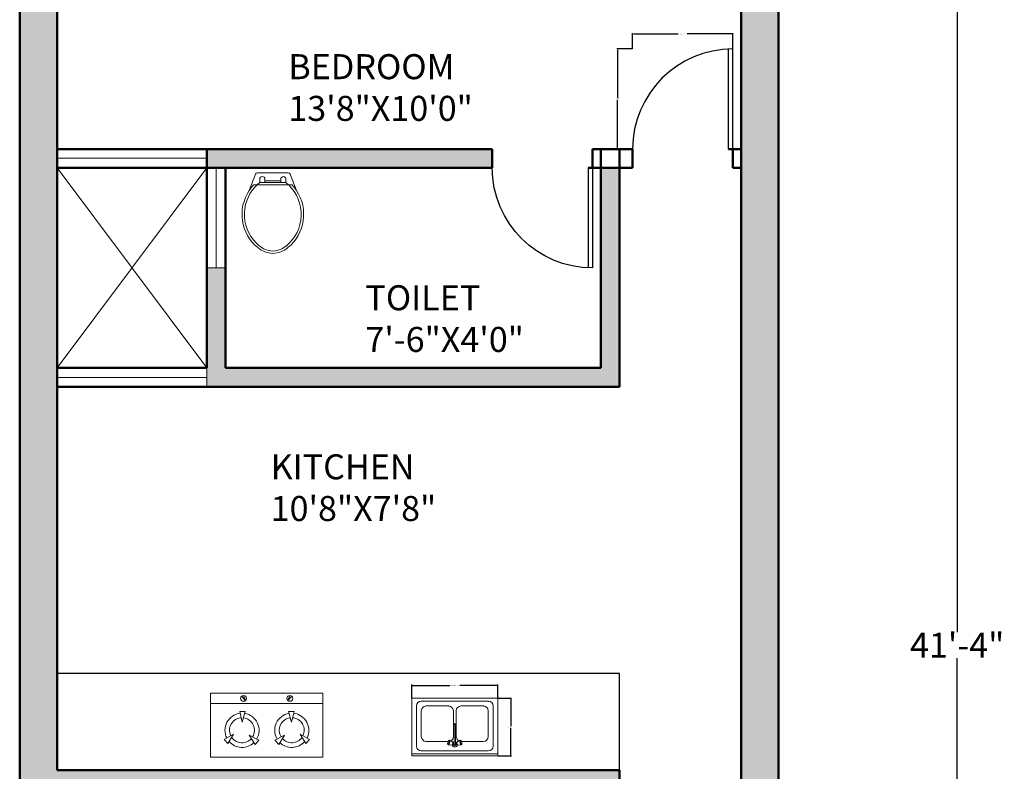
# Model space of a CAD drawing. Units: inches. Extents: x 3 to 485, y -522 to 42.
# Tile 5 of 6: x 249 to 485, y -264 to -84. Entities that reach past the tile are written whole.
import ezdxf

# ---------------------------------------------------------------- set-up
doc = ezdxf.new("R2010")
doc.units = ezdxf.units.IN
doc.header["$MEASUREMENT"] = 0
for name, color, linetype, lineweight in [('A-ANNO-DIMS', 2, 'Continuous', 18), ('A-AREA-IDEN', 7, 'Continuous', 18), ('A-DOOR', 3, 'Continuous', 25), ('A-EQPM', 8, 'Continuous', 18), ('A-FLOR-CASE', 8, 'Continuous', 25), ('A-FLOR-FIXT', 9, 'Continuous', 18), ('A-FLOR-OPEN', 8, 'Continuous', 18), ('A-GLAZ', 4, 'Continuous', 18), ('A-WALL', 7, 'Continuous', 50)]:
    doc.layers.add(name, color=color, linetype=linetype, lineweight=lineweight)
doc.layers.add('A-WALL-PATT', color=18, linetype='Continuous', lineweight=13, true_color=0x000000)
doc.styles.get("Standard").update_dxf_attribs({"font": 'arial.ttf'})
doc.dimstyles.get("Standard").update_dxf_attribs({"dimtxt": 0.18, "dimasz": 0.18, "dimexe": 0.18, "dimexo": 0.0625, "dimgap": 0.09, "dimtad": 0, "dimtih": 1, "dimtoh": 1, "dimdec": 0, "dimzin": 0, "dimdsep": 46, "dimlunit": 3, "dimtxsty": 'Standard', "dimcen": 0.09, "dimadec": 0, "dimazin": 0, "dimtfac": 1, "dimtdec": 0, "dimtofl": 0, "dimtmove": 0, "dimatfit": 3, "dimfxl": 1, "dimtolj": 1, "dimtzin": 0, "dimarcsym": 0})

# ---------------------------------------------------------------- blocks, each defined once
blk = doc.blocks.new('М07 600х900')
for p, q in [((0, 600), (-900, 600)), ((-900, 0), (-900, 600)), ((-900, 0), (-900, 600)), ((0, 580), (-900, 580)), ((-800, 550), (-100, 550)), ((0, 0), (0, 600)), ((0, 0), (0, 600)), ((-850, 80), (-850, 500)), ((-750, 450), (-519, 450)), ((-525, 477), (-524, 480)), ((-525, 472), (-525, 477)), ((-524, 466), (-525, 472)), ((-521, 486), (-524, 480)), ((-524, 480), (-522, 481)), ((-523, 460), (-524, 466)), ((-521, 455), (-523, 460)), ((-522, 481), (-520, 481)), ((-521, 486), (-519, 487)), ((-519, 449), (-521, 455)), ((-520, 481), (-518, 479)), ((-480, 488), (-519, 487)), ((-519, 487), (-516, 487)), ((-516, 445), (-519, 449)), ((-518, 479), (-515, 475)), ((-516, 487), (-513, 484)), ((-514, 443), (-516, 445)), ((-515, 475), (-513, 470)), ((-509, 440), (-514, 443)), ((-512, 443), (-514, 443)), ((-513, 484), (-510, 479)), ((-513, 470), (-511, 464)), ((-510, 444), (-512, 443)), ((-511, 464), (-510, 458)), ((-510, 479), (-507, 473)), ((-510, 458), (-509, 452)), ((-509, 447), (-510, 444)), ((-509, 452), (-509, 447)), ((-506, 439), (-509, 440)), ((-507, 473), (-505, 465)), ((-472, 459), (-506, 439)), ((-504, 441), (-506, 439)), ((-505, 465), (-503, 458)), ((-503, 445), (-504, 441)), ((-503, 458), (-503, 451)), ((-503, 451), (-503, 445)), ((-480, 488), (-478, 487)), ((-478, 487), (-476, 486)), ((-477, 489), (-473, 496)), ((-477, 486), (-477, 489)), ((-461, 489), (-476, 485)), ((-476, 486), (-474, 483)), ((-474, 483), (-473, 479)), ((-473, 496), (-466, 503)), ((-473, 479), (-471, 474)), ((-471, 460), (-472, 459)), ((-471, 474), (-470, 470)), ((-470, 462), (-471, 460)), ((-470, 470), (-470, 466)), ((-470, 466), (-470, 462)), ((-458, 465), (-470, 462)), ((-466, 457), (-470, 461)), ((-466, 503), (-459, 507)), ((-459, 453), (-466, 457)), ((-465, 480), (-462, 489)), ((-462, 471), (-465, 480)), ((-462, 489), (-455, 494)), ((-458, 469), (-462, 471)), ((-459, 507), (-450, 508)), ((-458, 453), (-459, 453)), ((-458, 480), (-457, 485)), ((-458, 480), (-458, 280)), ((-457, 485), (-453, 488)), ((-455, 494), (-445, 494)), ((-453, 488), (-447, 488)), ((-450, 508), (-441, 507)), ((-447, 488), (-443, 485)), ((-445, 494), (-438, 489)), ((-443, 485), (-442, 480)), ((-442, 480), (-442, 280)), ((-438, 471), (-442, 469)), ((-442, 465), (-430, 462)), ((-441, 453), (-442, 453)), ((-441, 507), (-434, 503)), ((-434, 457), (-441, 453)), ((-439, 489), (-424, 485)), ((-438, 489), (-435, 480)), ((-435, 480), (-438, 471)), ((-434, 503), (-427, 496)), ((-430, 461), (-434, 457)), ((-430, 470), (-429, 474)), ((-430, 466), (-430, 470)), ((-430, 462), (-430, 466)), ((-429, 460), (-430, 462)), ((-429, 474), (-427, 479)), ((-428, 459), (-429, 460)), ((-428, 459), (-394, 439)), ((-427, 496), (-423, 489)), ((-427, 479), (-426, 483)), ((-426, 483), (-424, 486)), ((-424, 486), (-422, 487)), ((-423, 489), (-423, 486)), ((-422, 487), (-420, 488)), ((-420, 488), (-381, 487)), ((-397, 458), (-395, 465)), ((-397, 451), (-397, 458)), ((-397, 445), (-397, 451)), ((-396, 441), (-397, 445)), ((-394, 439), (-396, 441)), ((-395, 465), (-393, 473)), ((-391, 440), (-394, 439)), ((-393, 473), (-390, 479)), ((-391, 452), (-390, 458)), ((-391, 447), (-391, 452)), ((-390, 444), (-391, 447)), ((-391, 440), (-386, 443)), ((-390, 479), (-387, 484)), ((-390, 458), (-389, 464)), ((-388, 443), (-390, 444)), ((-389, 464), (-387, 470)), ((-386, 443), (-388, 443)), ((-387, 484), (-384, 487)), ((-387, 470), (-385, 475)), ((-384, 445), (-386, 443)), ((-385, 475), (-382, 479)), ((-384, 487), (-381, 487)), ((-381, 449), (-384, 445)), ((-382, 479), (-380, 481)), ((-381, 487), (-379, 486)), ((-379, 455), (-381, 449)), ((-381, 450), (-150, 450)), ((-380, 481), (-378, 481)), ((-379, 486), (-376, 480)), ((-377, 460), (-379, 455)), ((-378, 481), (-376, 480)), ((-376, 466), (-377, 460)), ((-376, 480), (-375, 477)), ((-375, 472), (-376, 466)), ((-375, 477), (-375, 472)), ((-50, 500), (-50, 80)), ((-800, 130), (-800, 400)), ((-465, 400), (-465, 130)), ((-435, 130), (-435, 400)), ((-100, 400), (-100, 130)), ((-458, 286), (-460, 280)), ((-460, 280), (-458, 274)), ((-458, 280), (-457, 275)), ((-458, 274), (-457, 270)), ((-458, 274), (-453, 271)), ((-457, 275), (-453, 272)), ((-457, 270), (-453, 267)), ((-453, 272), (-447, 272)), ((-453, 271), (-447, 271)), ((-453, 267), (-447, 267)), ((-447, 272), (-443, 275)), ((-447, 271), (-442, 274)), ((-447, 267), (-443, 270)), ((-443, 275), (-442, 280)), ((-442, 274), (-443, 270)), ((-440, 280), (-442, 286)), ((-442, 274), (-440, 280)), ((0, 0), (-900, 0)), ((-100, 30), (-800, 30)), ((-515, 80), (-750, 80)), ((-150, 80), (-385, 80))]:
    blk.add_line(p, q)
for centre, start, end in [((-800, 500), 90, 180), ((-100, 500), 0, 90), ((-750, 400), 90, 180), ((-515, 400), 0, 65.8874), ((-385, 400), 114.1126, 180), ((-150, 400), 0, 90), ((-750, 130), 180, 270), ((-515, 130), 270, 0), ((-385, 130), 180, 270), ((-150, 130), 270, 0), ((-800, 80), 180, 270), ((-100, 80), 270, 0)]:
    blk.add_arc(centre, 50, start, end)
for p in [(-515, 80), (-150, 80), (-100, 30)]:
    blk.add_point(p)
blk = doc.blocks.new('*D7')
at = {"layer": 'A-ANNO-DIMS', "color": 0, "lineweight": -2, "transparency": 16777216}
for p, q in [((430.85, 14), (473.81, 14)), ((473.63, 13.82), (473.63, -230.89)), ((473.63, -481.82), (473.63, -237.1)), ((430.85, -482), (473.81, -482))]:
    blk.add_line(p, q, dxfattribs=at)
at = {"layer": 'A-ANNO-DIMS', "color": 0, "transparency": 16777216}
for points in [[(473.6, 13.82), (473.66, 13.82), (473.63, 14)], [(473.6, -481.82), (473.66, -481.82), (473.63, -482)]]:
    blk.add_solid(points, dxfattribs=at)
at = {"layer": 'Defpoints', "color": 0, "transparency": 16777216}
for p in [(430.79, 14), (430.79, -482), (473.63, -482)]:
    blk.add_point(p, dxfattribs=at)
at = {"layer": 'A-ANNO-DIMS', "color": 0, "transparency": 16777216, "insert": (473.63, -234), "char_height": 6, "attachment_point": 5}
blk.add_mtext('\\A1;41\'-4"', dxfattribs=at)
blk = doc.blocks.new('WC-PLAN')
for p, q in [((2.77, 16.42), (3.59, 16.42)), ((3.59, 16.42), (7.39, 16.42)), ((11.2, 16.42), (7.39, 16.42)), ((11.2, 16.42), (12.01, 16.42))]:
    blk.add_line(p, q)
for points in [[(7.39, 19.36), (3.7, 19.36, 0.31031), (3.24, 19.04), (1.73, 15.1, 0.209071)], [(7.39, 19.36), (11.09, 19.36, -0.31031), (11.54, 19.04), (13.06, 15.1, -0.209071)], [(4.25, 17.01, 0.022712), (3.59, 16.42, 0.162618)], [(4.25, 17.01), (4.25, 17.82, -1), (5.49, 17.82), (5.49, 17.4)], [(7.39, 17.01), (4.25, 17.01, 0.022712)], [(7.39, 17.01), (10.53, 17.01, -0.476108)], [(10.53, 17.01), (10.53, 17.82, 1), (9.3, 17.82), (9.3, 17.4)], [(10.53, 17.01, -0.022712), (11.2, 16.42, -0.162618)], [(1.73, 15.1, 0.383919), (3.76, 1.39, 0.163732), (7.39, 0, 0.359733)], [(3.2, 16.03, 0.431639), (4.12, 1.84, 0.162618), (7.39, 0.58, 0.470877)], [(2.77, 16.42, 0.040937), (1.73, 15.1, 0.163732)], [(3.59, 16.42, 0.014165), (3.2, 16.03, 0.162618)], [(11.2, 16.42, -0.448546), (10.66, 1.84, -0.162618), (7.39, 0.58, -0.470877)], [(13.06, 15.1, -0.383919), (11.03, 1.39, -0.163732), (7.39, 0, -0.359733)], [(12.01, 16.42, -0.040937), (13.06, 15.1, -0.163732)]]:
    blk.add_lwpolyline(points, format="xyb")
for points in [[(9.3, 17.4), (5.49, 17.4)], [(5.49, 17.4), (5.49, 17.01)], [(9.3, 17.4), (9.3, 17.01)]]:
    blk.add_lwpolyline(points)
blk = doc.blocks.new('COOKTOP-TWO-BURNER')
for p, q in [((4.16, 12.04), (3.23, 11.09)), ((5.52, 9.82), (4.16, 12.04)), ((10.65, 12.28), (9.27, 10.05)), ((11.55, 11.31), (10.65, 12.28)), ((15.42, 11.31), (16.32, 12.28)), ((16.32, 12.28), (17.71, 10.05)), ((21.45, 9.82), (22.81, 12.04)), ((22.81, 12.04), (23.74, 11.09)), ((3.23, 11.09), (5.52, 9.82)), ((9.27, 10.05), (11.55, 11.31)), ((17.71, 10.05), (15.42, 11.31)), ((23.74, 11.09), (21.45, 9.82)), ((7.59, 6.96), (6.96, 4.43)), ((8.29, 4.43), (7.59, 6.96)), ((18.68, 4.43), (19.38, 6.96)), ((19.38, 6.96), (20.01, 4.43)), ((26.9, 2.5), (0, 2.5)), ((6.96, 4.43), (8.29, 4.43)), ((20.01, 4.43), (18.68, 4.43))]:
    blk.add_line(p, q)
at = {"ltscale": 20}
for p, q in [((8.39, 1.74), (7.39, 0.75)), ((7.89, 0.54), (8.39, 1.74)), ((18.51, 1.74), (19.51, 0.75)), ((19.01, 0.54), (18.51, 1.74))]:
    blk.add_line(p, q, dxfattribs=at)
blk.add_lwpolyline([(0, 15.37), (26.9, 15.37), (26.9, 0), (0, 0)], close=True)
for centre in [(7.89, 1.25), (19.01, 1.25)]:
    blk.add_circle(centre, 0.707, dxfattribs=at)
for centre, radius, start, end in [((7.52, 8.9), 4.1, 45.8373, 138.7775), ((7.52, 8.9), 3, 41.1973, 145.4439), ((19.45, 8.9), 4.1, 41.2225, 134.1627), ((19.45, 8.9), 3, 34.5561, 138.8027), ((7.52, 8.9), 4.1, 153.231, 263.5995), ((7.52, 8.9), 3, 154.0793, 266.4247), ((7.52, 8.9), 3, 276.98, 32.0222), ((7.52, 8.9), 4.1, 279.2438, 31.147), ((19.45, 8.9), 4.1, 148.853, 260.7562), ((19.45, 8.9), 3, 147.9778, 263.02), ((19.45, 8.9), 3, 273.5753, 25.9207), ((19.45, 8.9), 4.1, 276.4005, 26.769)]:
    blk.add_arc(centre, radius, start, end)
blk = doc.blocks.new('DOOR-SWING-24IN')
for p, q in [((-1, 0), (-1, 24)), ((0, 0), (0, 24))]:
    blk.add_line(p, q)
blk.add_arc((0, 0), 24, 90, 180)
blk = doc.blocks.new('*D14')
at = {"layer": 'A-ANNO-DIMS', "color": 0, "lineweight": -2, "transparency": 16777216}
for p, q in [((395.79, -90.93), (395.79, -87.22)), ((419.79, -90.93), (419.79, -87.22)), ((395.97, -87.4), (406.74, -87.4)), ((419.61, -87.4), (408.84, -87.4))]:
    blk.add_line(p, q, dxfattribs=at)
at = {"layer": 'A-ANNO-DIMS', "color": 0, "transparency": 16777216}
for points in [[(395.97, -87.37), (395.97, -87.43), (395.79, -87.4)], [(419.61, -87.37), (419.61, -87.43), (419.79, -87.4)]]:
    blk.add_solid(points, dxfattribs=at)
at = {"layer": 'Defpoints', "color": 0, "transparency": 16777216}
for p in [(419.79, -87.4), (395.79, -91), (419.79, -91)]:
    blk.add_point(p, dxfattribs=at)
at = {"layer": 'A-ANNO-DIMS', "color": 0, "transparency": 16777216, "insert": (407.79, -87.4), "char_height": 0.18, "attachment_point": 5}
blk.add_mtext('\\A1;DOOR 2\'-0" TYP.', dxfattribs=at)
blk = doc.blocks.new('*D15')
at = {"layer": 'A-ANNO-DIMS', "color": 0, "lineweight": -2, "transparency": 16777216}
for p, q in [((395.73, -91), (392.01, -91)), ((392.19, -91.18), (392.19, -102.81)), ((392.19, -114.82), (392.19, -103.18)), ((395.73, -115), (392.01, -115))]:
    blk.add_line(p, q, dxfattribs=at)
at = {"layer": 'A-ANNO-DIMS', "color": 0, "transparency": 16777216}
for points in [[(392.16, -91.18), (392.22, -91.18), (392.19, -91)], [(392.16, -114.82), (392.22, -114.82), (392.19, -115)]]:
    blk.add_solid(points, dxfattribs=at)
at = {"layer": 'Defpoints', "color": 0, "transparency": 16777216}
for p in [(392.19, -91), (395.79, -91), (395.79, -115)]:
    blk.add_point(p, dxfattribs=at)
at = {"layer": 'A-ANNO-DIMS', "color": 0, "transparency": 16777216, "insert": (392.19, -103), "char_height": 0.18, "attachment_point": 5}
blk.add_mtext('\\A1;2\'-0" TYP.', dxfattribs=at)
blk = doc.blocks.new('*D16')
at = {"layer": 'A-ANNO-DIMS', "color": 0, "lineweight": -2, "transparency": 16777216}
for p, q in [((342.81, -246.67), (342.81, -243.45)), ((342.99, -243.63), (351.97, -243.63)), ((363.3, -243.63), (354.32, -243.63)), ((363.48, -246.67), (363.48, -243.45))]:
    blk.add_line(p, q, dxfattribs=at)
at = {"layer": 'A-ANNO-DIMS', "color": 0, "transparency": 16777216}
for points in [[(342.99, -243.6), (342.99, -243.66), (342.81, -243.63)], [(363.3, -243.6), (363.3, -243.66), (363.48, -243.63)]]:
    blk.add_solid(points, dxfattribs=at)
at = {"layer": 'Defpoints', "color": 0, "transparency": 16777216}
for p in [(363.48, -243.63), (342.81, -246.73), (363.48, -246.73)]:
    blk.add_point(p, dxfattribs=at)
at = {"layer": 'A-ANNO-DIMS', "color": 0, "transparency": 16777216, "insert": (353.14, -243.63), "char_height": 0.18, "attachment_point": 5}
blk.add_mtext('\\A1;SINK 1\'-8 1/2" TYP.', dxfattribs=at)
blk = doc.blocks.new('*D17')
at = {"layer": 'A-ANNO-DIMS', "color": 0, "lineweight": -2, "transparency": 16777216}
for p, q in [((363.54, -246.73), (366.76, -246.73)), ((366.58, -246.91), (366.58, -253.44)), ((366.58, -260.33), (366.58, -253.8)), ((363.54, -260.51), (366.76, -260.51))]:
    blk.add_line(p, q, dxfattribs=at)
at = {"layer": 'A-ANNO-DIMS', "color": 0, "transparency": 16777216}
for points in [[(366.55, -246.91), (366.61, -246.91), (366.58, -246.73)], [(366.55, -260.33), (366.61, -260.33), (366.58, -260.51)]]:
    blk.add_solid(points, dxfattribs=at)
at = {"layer": 'Defpoints', "color": 0, "transparency": 16777216}
for p in [(363.48, -246.73), (363.48, -260.51), (366.58, -260.51)]:
    blk.add_point(p, dxfattribs=at)
at = {"layer": 'A-ANNO-DIMS', "color": 0, "transparency": 16777216, "insert": (366.58, -253.62), "char_height": 0.18, "attachment_point": 5}
blk.add_mtext('\\A1;1\'-2" TYP.', dxfattribs=at)

msp = doc.modelspace()

# ---------------------------------------------------------------- hatches: boundary and pattern name
at = {"layer": 'A-WALL-PATT'}
h = msp.add_hatch(color=256, dxfattribs=at)
h.dxf.hatch_style = 1
h.paths.add_polyline_path([(257.79, 5), (421.79, 5), (421.79, -482), (430.79, -482), (430.79, 14), (248.79, 14), (248.79, -482), (257.79, -482), (257.79, -393), (311.15, -393), (311.15, -388.5), (257.79, -388.5), (257.79, -268.5), (392.64, -268.5), (392.64, -264), (257.79, -264)])
h.paths.add_polyline_path([(358.77, -482), (358.77, -473), (298.77, -473), (298.77, -482)], flags=17)
h.paths.add_polyline_path([(298.14, -167.5), (298.14, -143.5), (293.64, -143.5), (293.64, -167.5), (293.64, -172), (392.64, -172), (392.64, -167.5), (392.64, -119.5), (388.14, -119.5), (388.14, -167.5)], flags=17)
h.paths.add_polyline_path([(362.14, -119.5), (362.14, -115), (293.64, -115), (293.64, -119.5)], flags=17)

# ---------------------------------------------------------------- linework, layer by layer
at = {"layer": 'A-FLOR-CASE'}
for p, q in [((392.64, -240.77), (257.79, -240.77)), ((392.64, -264), (392.64, -240.77))]:
    msp.add_line(p, q, dxfattribs=at)
at = {"layer": 'A-FLOR-OPEN'}
for p, q in [((257.79, -119.5), (293.64, -167.5)), ((293.64, -119.5), (257.79, -167.5))]:
    msp.add_line(p, q, dxfattribs=at)
at = {"layer": 'A-GLAZ'}
for p, q in [((257.79, -117.2), (293.64, -117.2)), ((295.89, -143.5), (295.89, -119.5)), ((298.14, -143.5), (293.64, -143.5)), ((293.64, -167.5), (293.64, -172)), ((293.64, -169.75), (257.79, -169.75))]:
    msp.add_line(p, q, dxfattribs=at)
at = {"layer": 'A-WALL'}
for p, q in [((248.79, 14), (248.79, -482)), ((430.79, 14), (430.79, -482)), ((257.79, 5), (257.79, -264)), ((421.79, 5), (421.79, -482)), ((257.79, -115), (362.14, -115)), ((293.64, -115), (293.64, -167.5)), ((362.14, -119.5), (362.14, -115)), ((386.14, -115), (386.14, -119.5)), ((386.14, -115), (395.79, -115)), ((388.14, -115), (388.14, -167.5)), ((392.64, -115), (392.64, -167.5)), ((395.79, -119.5), (395.79, -115)), ((418.79, -115), (421.79, -115)), ((419.79, -119.5), (419.79, -115)), ((257.79, -119.5), (362.14, -119.5)), ((298.14, -119.5), (298.14, -167.5)), ((385.14, -119.5), (395.79, -119.5)), ((419.79, -119.5), (421.79, -119.5)), ((257.79, -167.5), (293.64, -167.5)), ((298.14, -167.5), (388.14, -167.5)), ((392.64, -167.5), (392.64, -172)), ((257.79, -172), (392.64, -172)), ((257.79, -264), (392.64, -264)), ((392.64, -264), (392.64, -268.5))]:
    msp.add_line(p, q, dxfattribs=at)

# ---------------------------------------------------------------- block references
at = {"layer": 'A-DOOR'}
msp.add_blockref('DOOR-SWING-24IN', (419.79, -115), dxfattribs=at)
at = {"layer": 'A-DOOR', "extrusion": (0, 0, -1), "zscale": -1, "rotation": 180}
msp.add_blockref('DOOR-SWING-24IN', (-386.14, -119.5), dxfattribs=at)
at = {"layer": 'A-EQPM', "extrusion": (0, 0, -1), "zscale": -1, "rotation": 180}
msp.add_blockref('COOKTOP-TWO-BURNER', (-294.59, -245.5), dxfattribs=at)
at = {"layer": 'A-FLOR-FIXT'}
msp.add_blockref('WC-PLAN', (302.11, -140.04), dxfattribs=at)
at = {"layer": 'A-FLOR-FIXT', "xscale": -0.0229615710193718, "yscale": 0.0229615710193718, "zscale": 0.0229615710193718, "rotation": 180}
msp.add_blockref('М07 600х900', (363.48, -246.73), dxfattribs=at)

# ---------------------------------------------------------------- texts
at = {"layer": 'A-AREA-IDEN', "char_height": 6, "attachment_point": 1}
for s, insert in [('BEDROOM\\P13\'8"X10\'0"', (313.22, -92.24)), ('TOILET\\P7\'-6"X4\'0"', (331.71, -147.66)), ('KITCHEN\\P10\'8"X7\'8"', (308.98, -188.21))]:
    msp.add_mtext(s, dxfattribs=dict(at, insert=insert))

# ---------------------------------------------------------------- dimensions: what is measured, and where the dimension line sits
at = {"layer": 'A-ANNO-DIMS'}
dim = msp.add_linear_dim(base=(473.63, -482), p1=(430.79, 14), p2=(430.79, -482), angle=90, dimstyle='Standard', override={"dimtxt": 6, "dimclrd": 0, "dimclre": 0, "dimclrt": 0}, dxfattribs=at)
dim.commit()
dim.dimension.update_dxf_attribs({"geometry": '*D7', "text_midpoint": (473.63, -234)})
for base, p1, p2, text, picture, middle in [((419.79, -87.4), (395.79, -91), (419.79, -91), 'DOOR <> TYP.', '*D14', (407.79, -87.4)), ((363.48, -243.63), (342.81, -246.73), (363.48, -246.73), 'SINK <> TYP.', '*D16', (353.14, -243.63))]:
    dim = msp.add_linear_dim(base=base, p1=p1, p2=p2, text=text, dimstyle='Standard', override={"dimdec": 1, "dimlfac": 1, "dimrnd": 0, "dimzin": 1, "dimdsep": 46, "dimlunit": 4, "dimfrac": 2}, dxfattribs=at)
    dim.commit()
    dim.dimension.update_dxf_attribs({"geometry": picture, "text_midpoint": middle})
for base, p1, p2, angle, picture, middle in [((392.19, -91), (395.79, -115), (395.79, -91), 90, '*D15', (392.19, -103)), ((366.58, -260.51), (363.48, -246.73), (363.48, -260.51), 270, '*D17', (366.58, -253.62))]:
    dim = msp.add_linear_dim(base=base, p1=p1, p2=p2, angle=angle, text='<> TYP.', dimstyle='Standard', override={"dimdec": 1, "dimlfac": 1, "dimrnd": 0, "dimzin": 1, "dimdsep": 46, "dimlunit": 4, "dimfrac": 2}, dxfattribs=at)
    dim.commit()
    dim.dimension.update_dxf_attribs({"geometry": picture, "text_midpoint": middle})

doc.saveas('drawing.dxf')
